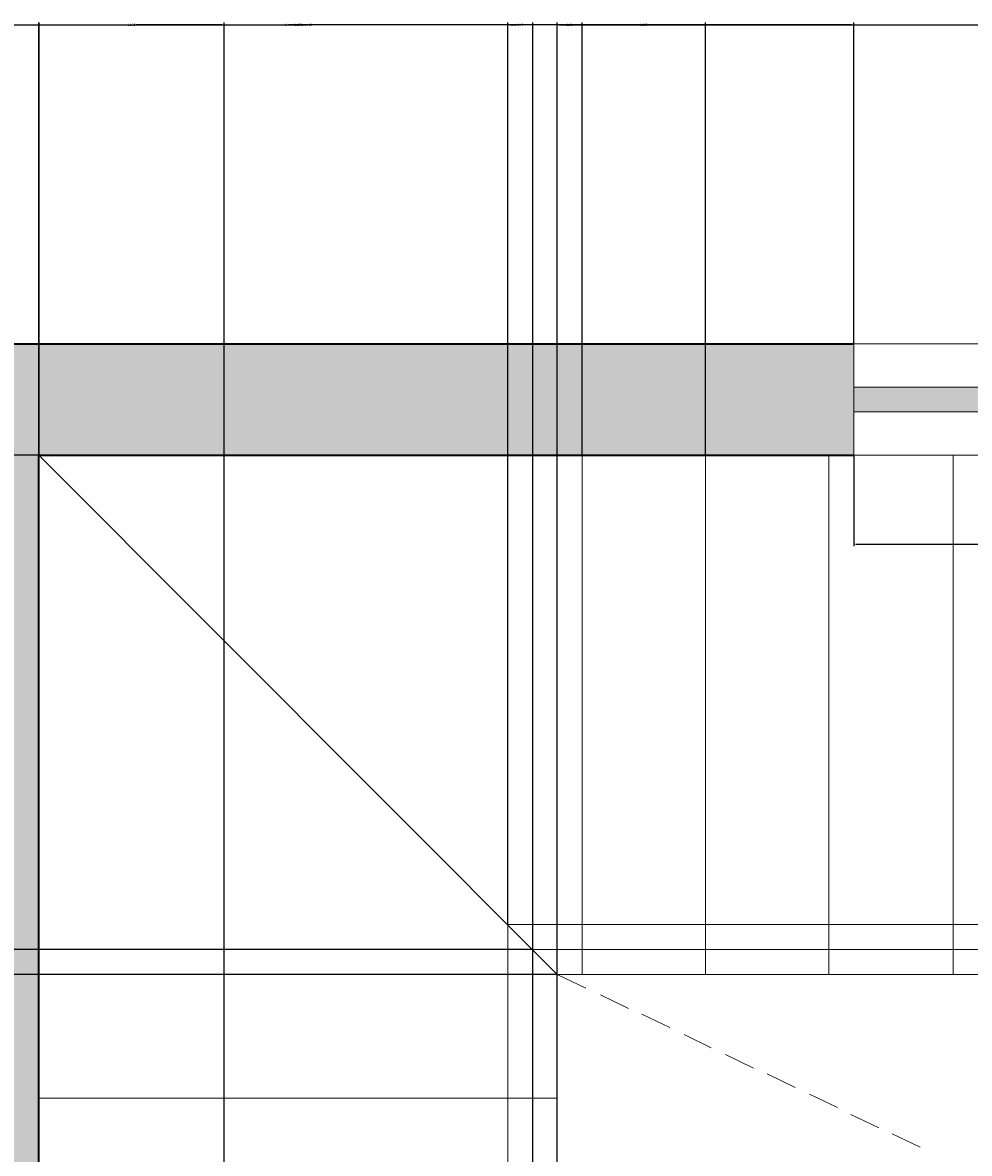
# Model space of a CAD drawing. Units: inches. Extents: x 6 to 575, y 34 to 566.
# Tile 12 of 21: x 205 to 282, y 474 to 566. Entities that reach past the tile are written whole.
import ezdxf

# ---------------------------------------------------------------- set-up
doc = ezdxf.new("R2010")
doc.units = ezdxf.units.IN
doc.linetypes.add('ACAD_ISO02W100', pattern=[15, 12, -3])
for name, color, linetype, lineweight in [('A-ANNO-DIMS', 2, 'Continuous', 18), ('A-FLOR-STRS-OVHD', 1, 'ACAD_ISO02W100', 13), ('A-GLAZ-PATT', 4, 'Continuous', 9), ('A-WALL-PATT', 251, 'Continuous', 9), ('STAIRS', 1, 'Continuous', 20), ('WALLS', 7, 'Continuous', 35), ('WINDOWS', 4, 'Continuous', 20)]:
    doc.layers.add(name, color=color, linetype=linetype, lineweight=lineweight)
doc.styles.get("Standard").update_dxf_attribs({"font": 'arial.ttf'})
doc.dimstyles.get("Standard").update_dxf_attribs({"dimtxt": 0.18, "dimasz": 0.18, "dimexe": 0.18, "dimexo": 0.0625, "dimgap": 0.09, "dimtad": 0, "dimtih": 1, "dimtoh": 1, "dimdec": 4, "dimzin": 0, "dimdsep": 46, "dimtxsty": 'Standard', "dimcen": 0.09, "dimadec": 0, "dimazin": 0, "dimtfac": 1, "dimtdec": 4, "dimtofl": 0, "dimtmove": 0, "dimatfit": 3, "dimfxl": 1, "dimtolj": 1, "dimtzin": 0, "dimarcsym": 0})

# ---------------------------------------------------------------- blocks, each defined once
blk = doc.blocks.new('WIN-48IN')
for p, q in [((0, 0), (0, 9)), ((0, 0), (0, 9)), ((0, 9), (0, 0)), ((48, 0), (48, 9)), ((0, 5.5), (48, 5.5)), ((0, 3.5), (48, 3.5))]:
    blk.add_line(p, q)
blk.add_lwpolyline([(0, 9), (48, 9), (48, 0), (0, 0)], close=True)
blk = doc.blocks.new('*D21')
at = {"layer": 'A-ANNO-DIMS', "color": 0, "lineweight": -2, "transparency": 16777216}
for p, q in [((272.659, 530.738), (272.659, 523.421)), ((320.659, 530.738), (320.659, 523.421)), ((272.839, 523.601), (295.54, 523.601)), ((320.479, 523.601), (297.777, 523.601))]:
    blk.add_line(p, q, dxfattribs=at)
at = {"layer": 'A-ANNO-DIMS', "color": 0, "transparency": 16777216}
for points in [[(272.839, 523.631), (272.839, 523.571), (272.659, 523.601)], [(320.479, 523.631), (320.479, 523.571), (320.659, 523.601)]]:
    blk.add_solid(points, dxfattribs=at)
at = {"layer": 'Defpoints', "color": 0, "transparency": 16777216}
for p in [(272.659, 530.801), (320.659, 530.801), (320.659, 523.601)]:
    blk.add_point(p, dxfattribs=at)
at = {"layer": 'A-ANNO-DIMS', "color": 0, "transparency": 16777216, "insert": (296.659, 523.601), "char_height": 0.18, "attachment_point": 5}
blk.add_mtext('\\A1;WINDOW 48 TYP.', dxfattribs=at)
blk = doc.blocks.new('*D33')
at = {"layer": 'A-ANNO-DIMS', "color": 0, "lineweight": -2, "transparency": 16777216}
for p, q in [((184.659, 539.863), (184.659, 565.811)), ((272.659, 539.863), (272.659, 565.811)), ((184.839, 565.631), (228.439, 565.631)), ((272.479, 565.631), (228.878, 565.631))]:
    blk.add_line(p, q, dxfattribs=at)
at = {"layer": 'A-ANNO-DIMS', "color": 0, "transparency": 16777216}
for points in [[(184.839, 565.661), (184.839, 565.601), (184.659, 565.631)], [(272.479, 565.661), (272.479, 565.601), (272.659, 565.631)]]:
    blk.add_solid(points, dxfattribs=at)
at = {"layer": 'Defpoints', "color": 0, "transparency": 16777216}
for p in [(272.659, 565.631), (184.659, 539.801), (272.659, 539.801)]:
    blk.add_point(p, dxfattribs=at)
at = {"layer": 'A-ANNO-DIMS', "color": 0, "transparency": 16777216, "insert": (228.659, 565.631), "char_height": 0.18, "attachment_point": 5}
blk.add_mtext('\\A1;88', dxfattribs=at)
blk = doc.blocks.new('*D49')
at = {"layer": 'A-ANNO-DIMS', "color": 0, "lineweight": -2, "transparency": 16777216}
for p, q in [((206.659, 448.865), (206.659, 565.811)), ((248.633, 448.865), (248.633, 565.811)), ((206.839, 565.631), (227.178, 565.631)), ((248.453, 565.631), (228.114, 565.631))]:
    blk.add_line(p, q, dxfattribs=at)
at = {"layer": 'A-ANNO-DIMS', "color": 0, "transparency": 16777216}
for points in [[(206.839, 565.661), (206.839, 565.601), (206.659, 565.631)], [(248.453, 565.661), (248.453, 565.601), (248.633, 565.631)]]:
    blk.add_solid(points, dxfattribs=at)
at = {"layer": 'Defpoints', "color": 0, "transparency": 16777216}
for p in [(248.633, 565.631), (206.659, 448.802), (248.633, 448.802)]:
    blk.add_point(p, dxfattribs=at)
at = {"layer": 'A-ANNO-DIMS', "color": 0, "transparency": 16777216, "insert": (227.646, 565.631), "char_height": 0.18, "attachment_point": 5}
blk.add_mtext('\\A1;41.975', dxfattribs=at)
blk = doc.blocks.new('*D59')
at = {"layer": 'A-ANNO-DIMS', "color": 0, "lineweight": -2, "transparency": 16777216}
for p, q in [((206.659, 224.863), (206.659, 565.811)), ((246.659, 224.863), (246.659, 565.811)), ((206.839, 565.631), (226.436, 565.631)), ((246.479, 565.631), (226.881, 565.631))]:
    blk.add_line(p, q, dxfattribs=at)
at = {"layer": 'A-ANNO-DIMS', "color": 0, "transparency": 16777216}
for points in [[(206.839, 565.661), (206.839, 565.601), (206.659, 565.631)], [(246.479, 565.661), (246.479, 565.601), (246.659, 565.631)]]:
    blk.add_solid(points, dxfattribs=at)
at = {"layer": 'Defpoints', "color": 0, "transparency": 16777216}
for p in [(246.659, 565.631), (206.659, 224.801), (246.659, 224.801)]:
    blk.add_point(p, dxfattribs=at)
at = {"layer": 'A-ANNO-DIMS', "color": 0, "transparency": 16777216, "insert": (226.659, 565.631), "char_height": 0.18, "attachment_point": 5}
blk.add_mtext('\\A1;40', dxfattribs=at)
blk = doc.blocks.new('*D68')
at = {"layer": 'A-ANNO-DIMS', "color": 0, "lineweight": -2, "transparency": 16777216}
for p, q in [((206.596, 530.801), (6.649, 530.801)), ((6.829, 530.621), (6.829, 509.957)), ((6.829, 488.928), (6.829, 509.593)), ((248.571, 488.748), (6.649, 488.748))]:
    blk.add_line(p, q, dxfattribs=at)
at = {"layer": 'A-ANNO-DIMS', "color": 0, "transparency": 16777216}
for points in [[(6.799, 530.621), (6.859, 530.621), (6.829, 530.801)], [(6.799, 488.928), (6.859, 488.928), (6.829, 488.748)]]:
    blk.add_solid(points, dxfattribs=at)
at = {"layer": 'Defpoints', "color": 0, "transparency": 16777216}
for p in [(206.659, 530.801), (6.829, 488.748), (248.633, 488.748)]:
    blk.add_point(p, dxfattribs=at)
at = {"layer": 'A-ANNO-DIMS', "color": 0, "transparency": 16777216, "insert": (6.829, 509.775), "char_height": 0.18, "attachment_point": 5}
blk.add_mtext('\\A1;42.05', dxfattribs=at)
blk = doc.blocks.new('*D69')
at = {"layer": 'A-ANNO-DIMS', "color": 0, "lineweight": -2, "transparency": 16777216}
for p, q in [((250.662, 530.863), (250.662, 565.811)), ((260.648, 530.863), (260.648, 565.811)), ((250.842, 565.631), (255.261, 565.631)), ((260.468, 565.631), (256.049, 565.631))]:
    blk.add_line(p, q, dxfattribs=at)
at = {"layer": 'A-ANNO-DIMS', "color": 0, "transparency": 16777216}
for points in [[(250.842, 565.661), (250.842, 565.601), (250.662, 565.631)], [(260.468, 565.661), (260.468, 565.601), (260.648, 565.631)]]:
    blk.add_solid(points, dxfattribs=at)
at = {"layer": 'Defpoints', "color": 0, "transparency": 16777216}
for p in [(260.648, 565.631), (250.662, 530.801), (260.648, 530.801)]:
    blk.add_point(p, dxfattribs=at)
at = {"layer": 'A-ANNO-DIMS', "color": 0, "transparency": 16777216, "insert": (255.655, 565.631), "char_height": 0.18, "attachment_point": 5}
blk.add_mtext('\\A1;9.987', dxfattribs=at)
blk = doc.blocks.new('*D70')
at = {"layer": 'A-ANNO-DIMS', "color": 0, "lineweight": -2, "transparency": 16777216}
for p, q in [((244.654, 492.868), (244.654, 565.811)), ((246.683, 490.839), (246.683, 565.811)), ((244.834, 565.631), (245.343, 565.631)), ((246.503, 565.631), (245.994, 565.631))]:
    blk.add_line(p, q, dxfattribs=at)
at = {"layer": 'A-ANNO-DIMS', "color": 0, "transparency": 16777216}
for points in [[(244.834, 565.661), (244.834, 565.601), (244.654, 565.631)], [(246.503, 565.661), (246.503, 565.601), (246.683, 565.631)]]:
    blk.add_solid(points, dxfattribs=at)
at = {"layer": 'Defpoints', "color": 0, "transparency": 16777216}
for p in [(246.683, 565.631), (244.654, 492.805), (246.683, 490.777)]:
    blk.add_point(p, dxfattribs=at)
at = {"layer": 'A-ANNO-DIMS', "color": 0, "transparency": 16777216, "insert": (245.668, 565.631), "char_height": 0.18, "attachment_point": 5}
blk.add_mtext('\\A1;2.03', dxfattribs=at)
blk = doc.blocks.new('*D71')
at = {"layer": 'A-ANNO-DIMS', "color": 0, "lineweight": -2, "transparency": 16777216}
for p, q in [((246.62, 490.777), (6.649, 490.777)), ((6.829, 490.597), (6.829, 489.945)), ((6.829, 488.928), (6.829, 489.581)), ((248.571, 488.748), (6.649, 488.748))]:
    blk.add_line(p, q, dxfattribs=at)
at = {"layer": 'A-ANNO-DIMS', "color": 0, "transparency": 16777216}
for points in [[(6.799, 490.597), (6.859, 490.597), (6.829, 490.777)], [(6.799, 488.928), (6.859, 488.928), (6.829, 488.748)]]:
    blk.add_solid(points, dxfattribs=at)
at = {"layer": 'Defpoints', "color": 0, "transparency": 16777216}
for p in [(246.683, 490.777), (6.829, 488.748), (248.633, 488.748)]:
    blk.add_point(p, dxfattribs=at)
at = {"layer": 'A-ANNO-DIMS', "color": 0, "transparency": 16777216, "insert": (6.829, 489.763), "char_height": 0.18, "attachment_point": 5}
blk.add_mtext('\\A1;2.03', dxfattribs=at)
blk = doc.blocks.new('*D72')
at = {"layer": 'A-ANNO-DIMS', "color": 0, "lineweight": -2, "transparency": 16777216}
for p, q in [((248.633, 488.811), (248.633, 565.811)), ((250.662, 530.863), (250.662, 565.811)), ((248.813, 565.631), (249.322, 565.631)), ((250.482, 565.631), (249.973, 565.631))]:
    blk.add_line(p, q, dxfattribs=at)
at = {"layer": 'A-ANNO-DIMS', "color": 0, "transparency": 16777216}
for points in [[(248.813, 565.661), (248.813, 565.601), (248.633, 565.631)], [(250.482, 565.661), (250.482, 565.601), (250.662, 565.631)]]:
    blk.add_solid(points, dxfattribs=at)
at = {"layer": 'Defpoints', "color": 0, "transparency": 16777216}
for p in [(250.662, 565.631), (250.662, 530.801), (248.633, 488.748)]:
    blk.add_point(p, dxfattribs=at)
at = {"layer": 'A-ANNO-DIMS', "color": 0, "transparency": 16777216, "insert": (249.647, 565.631), "char_height": 0.18, "attachment_point": 5}
blk.add_mtext('\\A1;2.03', dxfattribs=at)
blk = doc.blocks.new('*D73')
at = {"layer": 'A-ANNO-DIMS', "color": 0, "lineweight": -2, "transparency": 16777216}
for p, q in [((248.633, 448.865), (248.633, 565.811)), ((322.659, 448.863), (322.659, 565.811)), ((248.813, 565.631), (285.253, 565.631)), ((322.479, 565.631), (286.039, 565.631))]:
    blk.add_line(p, q, dxfattribs=at)
at = {"layer": 'A-ANNO-DIMS', "color": 0, "transparency": 16777216}
for points in [[(248.813, 565.661), (248.813, 565.601), (248.633, 565.631)], [(322.479, 565.661), (322.479, 565.601), (322.659, 565.631)]]:
    blk.add_solid(points, dxfattribs=at)
at = {"layer": 'Defpoints', "color": 0, "transparency": 16777216}
for p in [(322.659, 565.631), (248.633, 448.802), (322.659, 448.801)]:
    blk.add_point(p, dxfattribs=at)
at = {"layer": 'A-ANNO-DIMS', "color": 0, "transparency": 16777216, "insert": (285.646, 565.631), "char_height": 0.18, "attachment_point": 5}
blk.add_mtext('\\A1;74.03', dxfattribs=at)
blk = doc.blocks.new('*D135')
at = {"layer": 'A-ANNO-DIMS', "color": 0, "lineweight": -2, "transparency": 16777216}
for p, q in [((206.682, 389.512), (206.682, 565.811)), ((221.662, 389.512), (221.662, 565.811)), ((206.862, 565.631), (213.787, 565.631)), ((221.482, 565.631), (214.558, 565.631))]:
    blk.add_line(p, q, dxfattribs=at)
at = {"layer": 'A-ANNO-DIMS', "color": 0, "transparency": 16777216}
for points in [[(206.862, 565.661), (206.862, 565.601), (206.682, 565.631)], [(221.482, 565.661), (221.482, 565.601), (221.662, 565.631)]]:
    blk.add_solid(points, dxfattribs=at)
at = {"layer": 'Defpoints', "color": 0, "transparency": 16777216}
for p in [(221.662, 565.631), (206.682, 389.449), (221.662, 389.449)]:
    blk.add_point(p, dxfattribs=at)
at = {"layer": 'A-ANNO-DIMS', "color": 0, "transparency": 16777216, "insert": (214.172, 565.631), "char_height": 0.18, "attachment_point": 5}
blk.add_mtext('\\A1;14.98', dxfattribs=at)

msp = doc.modelspace()

# ---------------------------------------------------------------- hatches: boundary and pattern name
at = {"layer": 'A-GLAZ-PATT'}
h = msp.add_hatch(color=256, dxfattribs=at)
h.dxf.hatch_style = 1
h.paths.add_polyline_path([(36.1586, 224.801), (38.1586, 224.801), (38.1586, 272.801), (36.1586, 272.801)])
h.paths.add_polyline_path([(167.6586, 207.301), (167.6586, 209.301), (71.6586, 209.301), (71.6586, 207.301)])
h.paths.add_polyline_path([(264.6586, 219.301), (264.6586, 221.301), (246.6586, 221.301), (246.6586, 219.301)])
h.paths.add_polyline_path([(316.6586, 221.301), (316.6586, 219.301), (334.6586, 219.301), (334.6586, 221.301)])
h.paths.add_polyline_path([(515.6586, 207.301), (515.6586, 209.301), (407.6586, 209.301), (407.6586, 207.301)])
h.paths.add_polyline_path([(543.1586, 270.801), (545.1586, 270.801), (545.1586, 366.801), (543.1586, 366.801)])
h.paths.add_polyline_path([(407.9436, 536.301), (407.9436, 534.301), (455.9436, 534.301), (455.9436, 536.301)])
h.paths.add_polyline_path([(272.6586, 536.301), (272.6586, 534.301), (320.6586, 534.301), (320.6586, 536.301)])
at = {"layer": 'A-WALL-PATT'}
h = msp.add_hatch(color=256, dxfattribs=at)
h.dxf.hatch_style = 1
h.paths.add_polyline_path([(160.6586, 539.801), (32.6586, 539.801), (32.6586, 272.801), (41.6586, 272.801), (41.6586, 286.0643), (41.6586, 358.0764), (41.6586, 379.0637), (41.6586, 407.7709), (41.6194, 407.7709), (41.6194, 431.801), (82.8918, 431.801), (82.8918, 440.801), (65.6494, 440.801), (65.6494, 440.7732), (41.6194, 440.7732), (41.6194, 515.5941), (41.6586, 530.801), (117.6586, 530.801), (117.6586, 474.801), (120.6068, 474.801), (121.6586, 474.801), (121.6586, 530.801), (137.4275, 530.801), (137.4275, 530.8356), (141.2505, 530.8356), (160.6586, 530.801)])
h.paths.add_polyline_path([(71.6586, 212.801), (41.6586, 212.801), (41.6586, 224.801), (32.6586, 224.801), (32.6586, 203.801), (71.6586, 203.801)])
h.paths.add_polyline_path([(206.6586, 215.801), (246.6586, 215.801), (246.6586, 224.801), (206.6586, 224.801), (206.6586, 230.801), (201.8157, 230.801), (197.6586, 230.801), (197.6586, 212.801), (167.6586, 212.801), (167.6586, 203.801), (206.6586, 203.801)])
h.paths.add_polyline_path([(383.6586, 224.801), (334.6586, 224.801), (334.6586, 215.801), (374.6586, 215.801), (374.6586, 203.801), (384.0753, 203.801), (407.6586, 203.801), (407.6586, 212.801), (383.6586, 212.801)])
h.paths.add_polyline_path([(548.6586, 270.801), (539.6586, 270.801), (539.6586, 212.801), (515.6586, 212.801), (515.6586, 203.801), (548.6586, 203.801)])
h.paths.add_polyline_path([(548.6586, 412.801), (545.7108, 412.801), (539.6586, 412.801), (539.6586, 382.801), (433.708, 382.801), (433.708, 378.801), (539.6586, 378.801), (539.6586, 366.801), (548.6586, 366.801)])
h.paths.add_polyline_path([(548.6586, 539.801), (455.9436, 539.801), (455.9436, 530.801), (539.6586, 530.801), (539.6586, 440.801), (548.6586, 440.801)])
h.paths.add_polyline_path([(407.9436, 539.801), (362.6586, 539.801), (362.6586, 530.801), (374.6586, 530.801), (374.6586, 452.801), (354.6586, 452.801), (354.6586, 448.801), (374.6586, 448.801), (374.6586, 278.801), (383.6586, 278.801), (383.6586, 530.801), (407.9436, 530.801)])
h.paths.add_polyline_path([(338.6586, 539.801), (320.6586, 539.801), (320.6586, 530.801), (322.6586, 530.801), (322.6586, 448.801), (326.6586, 448.801), (326.6586, 530.801), (338.6586, 530.801)])
h.paths.add_polyline_path([(272.6586, 539.801), (184.6586, 539.801), (184.6586, 530.801), (197.6586, 530.801), (197.6586, 440.801), (176.6714, 440.801), (121.6586, 440.801), (121.6586, 446.801), (117.6586, 446.801), (117.6586, 440.801), (111.6586, 440.801), (111.6586, 431.801), (197.6586, 431.801), (197.6586, 407.7709), (197.6586, 276.801), (206.6586, 276.801), (206.6586, 530.801), (272.6586, 530.801)])

# ---------------------------------------------------------------- linework, layer by layer
at = {"layer": 'A-FLOR-STRS-OVHD'}
for points in [[(248.6332, 488.7484), (250.9738, 487.6561)], [(252.1441, 487.11), (254.4067, 486.0177)], [(255.4989, 485.5496), (257.7615, 484.4573)], [(258.9318, 483.9112), (261.1163, 482.8189)], [(262.2866, 482.2728), (264.5492, 481.1805)], [(265.6415, 480.7124), (267.9041, 479.6201)], [(269.0743, 479.074), (271.3369, 477.9817)], [(272.4292, 477.4356), (274.6918, 476.3433)], [(275.784, 475.8752), (278.0466, 474.7829)]]:
    msp.add_lwpolyline(points, dxfattribs=at)
at = {"layer": 'STAIRS'}
for points in [[(206.6586, 448.8024), (248.6332, 448.8024), (248.6332, 488.7484), (206.6586, 530.801)], [(250.6617, 488.7484), (250.6617, 530.801)], [(320.6453, 530.801), (260.6482, 530.801)], [(260.6482, 488.7484), (260.6482, 530.801)], [(270.6347, 488.7484), (270.6347, 530.801)], [(280.6993, 488.7484), (280.6993, 530.801)], [(244.6542, 448.8024), (244.6542, 492.8054), (320.6453, 492.8054)], [(246.6827, 448.8024), (246.6827, 490.7769), (320.6453, 490.7769)], [(206.6586, 488.7484), (248.6332, 488.7484), (320.6453, 488.7484)], [(206.6586, 478.7619), (248.6332, 478.7619)]]:
    msp.add_lwpolyline(points, dxfattribs=at)
at = {"layer": 'WALLS'}
for p, q in [((184.6586, 539.801), (272.6586, 539.801)), ((206.6586, 530.801), (272.6586, 530.801)), ((206.6586, 276.801), (206.6586, 530.801))]:
    msp.add_line(p, q, dxfattribs=at)

# ---------------------------------------------------------------- block references
at = {"layer": 'WINDOWS'}
msp.add_blockref('WIN-48IN', (272.659, 530.801), dxfattribs=at)

# ---------------------------------------------------------------- dimensions: what is measured, and where the dimension line sits
at = {"layer": 'A-ANNO-DIMS'}
for base, p1, p2, override, picture, middle in [((272.6586, 565.631), (184.6586, 539.801), (272.6586, 539.801), {"dimdec": 0, "dimlfac": 1, "dimrnd": 0, "dimzin": 0, "dimdsep": 46, "dimlunit": 2}, '*D33', (228.6586, 565.631)), ((248.6332, 565.631), (206.6586, 448.8024), (248.6332, 448.8024), {"dimdec": 3, "dimlfac": 1, "dimrnd": 0, "dimzin": 0, "dimdsep": 46, "dimlunit": 2}, '*D49', (227.6459, 565.631)), ((246.6586, 565.631), (206.6586, 224.801), (246.6586, 224.801), {"dimdec": 0, "dimlfac": 1, "dimrnd": 0, "dimzin": 0, "dimdsep": 46, "dimlunit": 2}, '*D59', (226.6586, 565.631)), ((221.6622, 565.631), (206.6824, 389.449), (221.6622, 389.449), {"dimdec": 2, "dimlfac": 1, "dimrnd": 0, "dimzin": 0, "dimdsep": 46, "dimlunit": 2}, '*D135', (214.1723, 565.631)), ((246.6827, 565.631), (244.6542, 492.8054), (246.6827, 490.7769), {"dimdec": 2, "dimlfac": 1, "dimrnd": 0, "dimzin": 0, "dimdsep": 46, "dimlunit": 2}, '*D70', (245.6685, 565.631)), ((250.6617, 565.631), (248.6332, 488.7484), (250.6617, 530.801), {"dimdec": 2, "dimlfac": 1, "dimrnd": 0, "dimzin": 0, "dimdsep": 46, "dimlunit": 2}, '*D72', (249.6475, 565.631)), ((322.6586, 565.631), (248.6332, 448.8024), (322.6586, 448.801), {"dimdec": 2, "dimlfac": 1, "dimrnd": 0, "dimzin": 0, "dimdsep": 46, "dimlunit": 2}, '*D73', (285.6459, 565.631)), ((260.64823, 565.63098), (250.66171, 530.80098), (260.64823, 530.80098), {"dimdec": 3, "dimlfac": 1, "dimrnd": 0, "dimzin": 0, "dimdsep": 46, "dimlunit": 2}, '*D69', (255.65497, 565.63098))]:
    dim = msp.add_linear_dim(base=base, p1=p1, p2=p2, dimstyle='Standard', override=override, dxfattribs=at)
    dim.commit()
    dim.dimension.update_dxf_attribs({"geometry": picture, "text_midpoint": middle})
for p1, picture, middle in [((206.6586, 530.801), '*D68', (6.8286, 509.7747)), ((246.6827, 490.7769), '*D71', (6.8286, 489.7627))]:
    dim = msp.add_linear_dim(base=(6.8286, 488.7484), p1=p1, p2=(248.6332, 488.7484), angle=90, dimstyle='Standard', override={"dimdec": 2, "dimlfac": 1, "dimrnd": 0, "dimzin": 0, "dimdsep": 46, "dimlunit": 2}, dxfattribs=at)
    dim.commit()
    dim.dimension.update_dxf_attribs({"geometry": picture, "text_midpoint": middle})
dim = msp.add_linear_dim(base=(320.6586, 523.601), p1=(272.6586, 530.801), p2=(320.6586, 530.801), text='WINDOW <> TYP.', dimstyle='Standard', override={"dimdec": 0, "dimlfac": 1, "dimrnd": 0, "dimzin": 0, "dimdsep": 46, "dimlunit": 2}, dxfattribs=at)
dim.commit()
dim.dimension.update_dxf_attribs({"geometry": '*D21', "text_midpoint": (296.6586, 523.601)})

doc.saveas('drawing.dxf')
